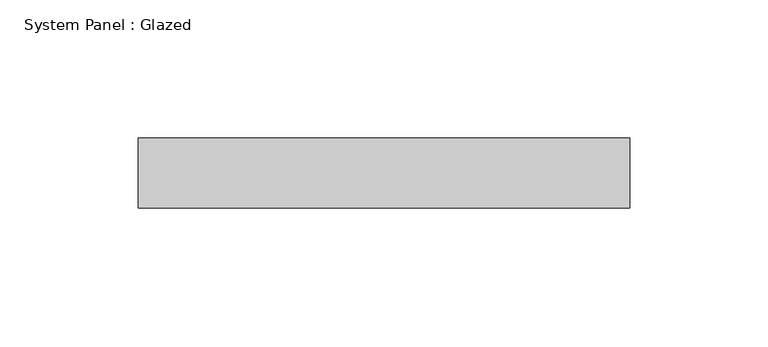
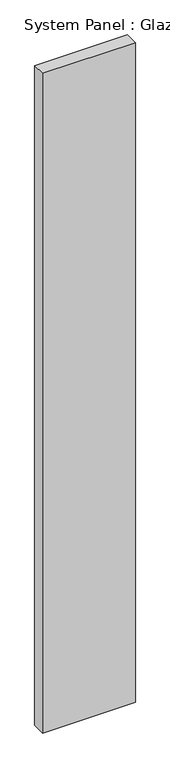
"""IFC4 building model written with IfcOpenShell, lengths in millimetres: plate geometry, System Panel : Glazed."""

from ifc_helpers import new_model, si_unit, origin, origin_with_axes, place, context, project, spatial, polyline, outline, extrude, source, transform, mapped, element, save


def system_panel_glazed_f8f6f98b(model_context):
    return source(origin(), model_context, "Body", "SweptSolid", [
        extrude(outline(polyline([(88.9, 19.05), (-88.9, 19.05), (-88.9, 44.45), (88.9, 44.45), (88.9, 19.05)])), origin_with_axes(), (0.0, 0.0, 1.0), 1333.5),
    ])


if __name__ == "__main__":
    model = new_model("IFC4")
    model_context = context("Model", 3, world=origin())
    ifc_project = project(units=[si_unit("LENGTHUNIT", "METRE", prefix="MILLI")], contexts=[model_context])
    site = spatial("IfcSite", under=ifc_project)
    building = spatial("IfcBuilding", under=site)
    placement = place(None, origin())
    system_panel_glazed_shape = system_panel_glazed_f8f6f98b(model_context)
    element("IfcPlate", 1, ObjectType="System Panel : Glazed", at=placement, inside=building, context=model_context, shape_type="MappedRepresentation", body=[
        mapped(system_panel_glazed_shape, transform((0.0, 0.0, 0.0), x_axis=(1.0, 0.0, 0.0), y_axis=(0.0, 1.0, 0.0), z_axis=(0.0, 0.0, 1.0))),
    ])
    save(model, "model.ifc")

# Revit data of these elements
# Type "System Panel : Glazed"
#   Construction Type Id = "GSP4R"
#   Analytic Construction = "1/8 in Pilkington single glazing"
#   Visual Light Transmittance = 0.9
#   Solar Heat Gain Coefficient = 0.86
#   Heat Transfer Coefficient (U) = 1.18115 BTU/(h·ft²·°F)
#   Define Thermal Properties by = 1
# Element 1 (IfcPlate, "System Panel : Glazed")
#   Materials on its faces: "Glass"
# Materials
#   "Glass": class "Glass", colour RGB 0 128 192, transparency 0.75, Description = "Soda Lime Glass", Cost = 0
